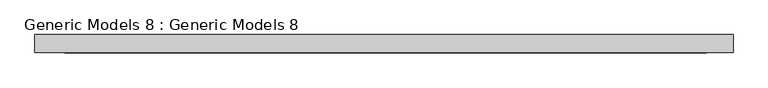
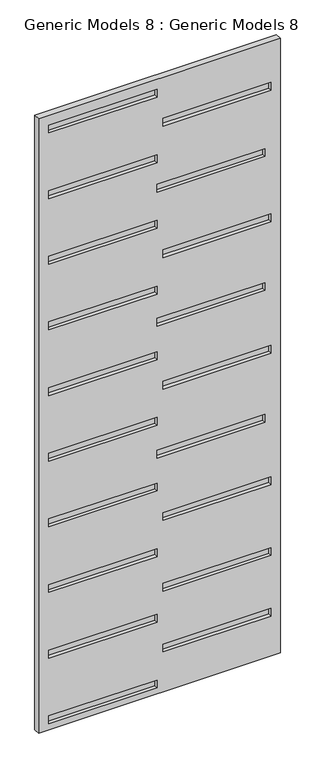
"""IFC4 building model written with IfcOpenShell, lengths in millimetres: proxy geometry, Generic Models 8 : Generic Models 8."""

from ifc_helpers import new_model, si_unit, origin, place, context, project, spatial, faceted_brep, source, transform, mapped, element, save


def generic_models_8_generic_models_8_98324a9d(model_context):
    return source(origin(), model_context, "Body", "Brep", [
        faceted_brep([(-3859.560819, -4187.674389, 7924.8), (-6812.6326914, -4187.674389, 7924.8), (-6812.6326914, -4187.674389, 0.0), (-3859.560819, -4187.674389, 0.0), (-5364.8326914, -4187.674389, 7797.8), (-5364.8326914, -4187.674389, 7696.2), (-6685.6326914, -4187.674389, 7696.2), (-6685.6326914, -4187.674389, 7797.8), (-5364.8326914, -4187.674389, 177.8), (-5364.8326914, -4187.674389, 76.2), (-6685.6326914, -4187.674389, 76.2), (-6685.6326914, -4187.674389, 177.8), (-5364.8326914, -4187.674389, 6951.1333333), (-5364.8326914, -4187.674389, 6849.5333333), (-6685.6326914, -4187.674389, 6849.5333333), (-6685.6326914, -4187.674389, 6951.1333333), (-5364.8326914, -4187.674389, 6104.4666667), (-5364.8326914, -4187.674389, 6002.8666667), (-6685.6326914, -4187.674389, 6002.8666667), (-6685.6326914, -4187.674389, 6104.4666667), (-5364.8326914, -4187.674389, 5257.8), (-5364.8326914, -4187.674389, 5156.2), (-6685.6326914, -4187.674389, 5156.2), (-6685.6326914, -4187.674389, 5257.8), (-5364.8326914, -4187.674389, 4411.1333333), (-5364.8326914, -4187.674389, 4309.5333333), (-6685.6326914, -4187.674389, 4309.5333333), (-6685.6326914, -4187.674389, 4411.1333333), (-5364.8326914, -4187.674389, 3564.4666667), (-5364.8326914, -4187.674389, 3462.8666667), (-6685.6326914, -4187.674389, 3462.8666667), (-6685.6326914, -4187.674389, 3564.4666667), (-5364.8326914, -4187.674389, 2717.8), (-5364.8326914, -4187.674389, 2616.2), (-6685.6326914, -4187.674389, 2616.2), (-6685.6326914, -4187.674389, 2717.8), (-5364.8326914, -4187.674389, 1871.1333333), (-5364.8326914, -4187.674389, 1769.5333333), (-6685.6326914, -4187.674389, 1769.5333333), (-6685.6326914, -4187.674389, 1871.1333333), (-5364.8326914, -4187.674389, 1024.4666667), (-5364.8326914, -4187.674389, 922.8666667), (-6685.6326914, -4187.674389, 922.8666667), (-6685.6326914, -4187.674389, 1024.4666667), (-3973.118008, -4187.674389, 7398.7322362), (-3973.118008, -4187.674389, 7297.1322362), (-5293.918008, -4187.674389, 7297.1322362), (-5293.918008, -4187.674389, 7398.7322362), (-3973.118008, -4187.674389, 616.9322362), (-3973.118008, -4187.674389, 515.3322362), (-5293.918008, -4187.674389, 515.3322362), (-5293.918008, -4187.674389, 616.9322362), (-3973.118008, -4187.674389, 5703.2822362), (-3973.118008, -4187.674389, 5601.6822362), (-5293.918008, -4187.674389, 5601.6822362), (-5293.918008, -4187.674389, 5703.2822362), (-3973.118008, -4187.674389, 4007.8322362), (-3973.118008, -4187.674389, 3906.2322362), (-5293.918008, -4187.674389, 3906.2322362), (-5293.918008, -4187.674389, 4007.8322362), (-3973.118008, -4187.674389, 2312.3822362), (-3973.118008, -4187.674389, 2210.7822362), (-5293.918008, -4187.674389, 2210.7822362), (-5293.918008, -4187.674389, 2312.3822362), (-4046.1719516, -4187.674389, 4842.8426322), (-4046.1719516, -4187.674389, 4741.2426322), (-5366.9719516, -4187.674389, 4741.2426322), (-5366.9719516, -4187.674389, 4842.8426322), (-4046.1719516, -4187.674389, 6570.0426322), (-4046.1719516, -4187.674389, 6468.4426322), (-5366.9719516, -4187.674389, 6468.4426322), (-5366.9719516, -4187.674389, 6570.0426322), (-4046.1719516, -4187.674389, 3141.0426322), (-4046.1719516, -4187.674389, 3039.4426322), (-5366.9719516, -4187.674389, 3039.4426322), (-5366.9719516, -4187.674389, 3141.0426322), (-3973.118008, -4187.674389, 1397.9822362), (-3973.118008, -4187.674389, 1296.3822362), (-5293.918008, -4187.674389, 1296.3822362), (-5293.918008, -4187.674389, 1397.9822362), (-3859.560819, -4111.474389, 7924.8), (-3859.560819, -4111.474389, 0.0), (-6812.6326914, -4111.474389, 0.0), (-6812.6326914, -4111.474389, 7924.8), (-5364.8326914, -4142.4938017, 7797.8), (-6685.6326914, -4142.4938017, 7797.8), (-6685.6326914, -4142.4938017, 7696.2), (-5364.8326914, -4142.4938017, 7696.2), (-5364.8326914, -4142.4938017, 177.8), (-6685.6326914, -4142.4938017, 177.8), (-6685.6326914, -4142.4938017, 76.2), (-5364.8326914, -4142.4938017, 76.2), (-5364.8326914, -4142.4938017, 6951.1333333), (-6685.6326914, -4142.4938017, 6951.1333333), (-6685.6326914, -4142.4938017, 6849.5333333), (-5364.8326914, -4142.4938017, 6849.5333333), (-5364.8326914, -4142.4938017, 6104.4666667), (-6685.6326914, -4142.4938017, 6104.4666667), (-6685.6326914, -4142.4938017, 6002.8666667), (-5364.8326914, -4142.4938017, 6002.8666667), (-5364.8326914, -4142.4938017, 5257.8), (-6685.6326914, -4142.4938017, 5257.8), (-6685.6326914, -4142.4938017, 5156.2), (-5364.8326914, -4142.4938017, 5156.2), (-5364.8326914, -4142.4938017, 4411.1333333), (-6685.6326914, -4142.4938017, 4411.1333333), (-6685.6326914, -4142.4938017, 4309.5333333), (-5364.8326914, -4142.4938017, 4309.5333333), (-5364.8326914, -4142.4938017, 3564.4666667), (-6685.6326914, -4142.4938017, 3564.4666667), (-6685.6326914, -4142.4938017, 3462.8666667), (-5364.8326914, -4142.4938017, 3462.8666667), (-5364.8326914, -4142.4938017, 2717.8), (-6685.6326914, -4142.4938017, 2717.8), (-6685.6326914, -4142.4938017, 2616.2), (-5364.8326914, -4142.4938017, 2616.2), (-5364.8326914, -4142.4938017, 1871.1333333), (-6685.6326914, -4142.4938017, 1871.1333333), (-6685.6326914, -4142.4938017, 1769.5333333), (-5364.8326914, -4142.4938017, 1769.5333333), (-5364.8326914, -4142.4938017, 1024.4666667), (-6685.6326914, -4142.4938017, 1024.4666667), (-6685.6326914, -4142.4938017, 922.8666667), (-5364.8326914, -4142.4938017, 922.8666667), (-3973.118008, -4142.4938017, 7398.7322362), (-5293.918008, -4142.4938017, 7398.7322362), (-5293.918008, -4142.4938017, 7297.1322362), (-3973.118008, -4142.4938017, 7297.1322362), (-3973.118008, -4142.4938017, 616.9322362), (-5293.918008, -4142.4938017, 616.9322362), (-5293.918008, -4142.4938017, 515.3322362), (-3973.118008, -4142.4938017, 515.3322362), (-3973.118008, -4142.4938017, 5703.2822362), (-5293.918008, -4142.4938017, 5703.2822362), (-5293.918008, -4142.4938017, 5601.6822362), (-3973.118008, -4142.4938017, 5601.6822362), (-3973.118008, -4142.4938017, 4007.8322362), (-5293.918008, -4142.4938017, 4007.8322362), (-5293.918008, -4142.4938017, 3906.2322362), (-3973.118008, -4142.4938017, 3906.2322362), (-3973.118008, -4142.4938017, 2312.3822362), (-5293.918008, -4142.4938017, 2312.3822362), (-5293.918008, -4142.4938017, 2210.7822362), (-3973.118008, -4142.4938017, 2210.7822362), (-4046.1719516, -4142.4938017, 4842.8426322), (-5366.9719516, -4142.4938017, 4842.8426322), (-5366.9719516, -4142.4938017, 4741.2426322), (-4046.1719516, -4142.4938017, 4741.2426322), (-4046.1719516, -4142.4938017, 6570.0426322), (-5366.9719516, -4142.4938017, 6570.0426322), (-5366.9719516, -4142.4938017, 6468.4426322), (-4046.1719516, -4142.4938017, 6468.4426322), (-4046.1719516, -4142.4938017, 3141.0426322), (-5366.9719516, -4142.4938017, 3141.0426322), (-5366.9719516, -4142.4938017, 3039.4426322), (-4046.1719516, -4142.4938017, 3039.4426322), (-3973.118008, -4142.4938017, 1397.9822362), (-5293.918008, -4142.4938017, 1397.9822362), (-5293.918008, -4142.4938017, 1296.3822362), (-3973.118008, -4142.4938017, 1296.3822362)], [[[0, 1, 2, 3], [4, 5, 6, 7], [8, 9, 10, 11], [12, 13, 14, 15], [16, 17, 18, 19], [20, 21, 22, 23], [24, 25, 26, 27], [28, 29, 30, 31], [32, 33, 34, 35], [36, 37, 38, 39], [40, 41, 42, 43], [44, 45, 46, 47], [48, 49, 50, 51], [52, 53, 54, 55], [56, 57, 58, 59], [60, 61, 62, 63], [64, 65, 66, 67], [68, 69, 70, 71], [72, 73, 74, 75], [76, 77, 78, 79]], [[80, 81, 82, 83]], [[1, 0, 80, 83]], [[2, 1, 83, 82]], [[3, 2, 82, 81]], [[0, 3, 81, 80]], [[84, 85, 86, 87]], [[84, 87, 5, 4]], [[87, 86, 6, 5]], [[86, 85, 7, 6]], [[85, 84, 4, 7]], [[88, 89, 90, 91]], [[88, 91, 9, 8]], [[91, 90, 10, 9]], [[90, 89, 11, 10]], [[89, 88, 8, 11]], [[92, 93, 94, 95]], [[92, 95, 13, 12]], [[95, 94, 14, 13]], [[94, 93, 15, 14]], [[93, 92, 12, 15]], [[96, 97, 98, 99]], [[96, 99, 17, 16]], [[99, 98, 18, 17]], [[98, 97, 19, 18]], [[97, 96, 16, 19]], [[100, 101, 102, 103]], [[100, 103, 21, 20]], [[103, 102, 22, 21]], [[102, 101, 23, 22]], [[101, 100, 20, 23]], [[104, 105, 106, 107]], [[104, 107, 25, 24]], [[107, 106, 26, 25]], [[106, 105, 27, 26]], [[105, 104, 24, 27]], [[108, 109, 110, 111]], [[108, 111, 29, 28]], [[111, 110, 30, 29]], [[110, 109, 31, 30]], [[109, 108, 28, 31]], [[112, 113, 114, 115]], [[112, 115, 33, 32]], [[115, 114, 34, 33]], [[114, 113, 35, 34]], [[113, 112, 32, 35]], [[116, 117, 118, 119]], [[116, 119, 37, 36]], [[119, 118, 38, 37]], [[118, 117, 39, 38]], [[117, 116, 36, 39]], [[120, 121, 122, 123]], [[120, 123, 41, 40]], [[123, 122, 42, 41]], [[122, 121, 43, 42]], [[121, 120, 40, 43]], [[124, 125, 126, 127]], [[124, 127, 45, 44]], [[127, 126, 46, 45]], [[126, 125, 47, 46]], [[125, 124, 44, 47]], [[128, 129, 130, 131]], [[128, 131, 49, 48]], [[131, 130, 50, 49]], [[130, 129, 51, 50]], [[129, 128, 48, 51]], [[132, 133, 134, 135]], [[132, 135, 53, 52]], [[135, 134, 54, 53]], [[134, 133, 55, 54]], [[133, 132, 52, 55]], [[136, 137, 138, 139]], [[136, 139, 57, 56]], [[139, 138, 58, 57]], [[138, 137, 59, 58]], [[137, 136, 56, 59]], [[140, 141, 142, 143]], [[140, 143, 61, 60]], [[143, 142, 62, 61]], [[142, 141, 63, 62]], [[141, 140, 60, 63]], [[144, 145, 146, 147]], [[144, 147, 65, 64]], [[147, 146, 66, 65]], [[146, 145, 67, 66]], [[145, 144, 64, 67]], [[148, 149, 150, 151]], [[148, 151, 69, 68]], [[151, 150, 70, 69]], [[150, 149, 71, 70]], [[149, 148, 68, 71]], [[152, 153, 154, 155]], [[152, 155, 73, 72]], [[155, 154, 74, 73]], [[154, 153, 75, 74]], [[153, 152, 72, 75]], [[156, 157, 158, 159]], [[156, 159, 77, 76]], [[159, 158, 78, 77]], [[158, 157, 79, 78]], [[157, 156, 76, 79]]]),
    ])


if __name__ == "__main__":
    model = new_model("IFC4")
    model_context = context("Model", 3, world=origin())
    ifc_project = project(units=[si_unit("LENGTHUNIT", "METRE", prefix="MILLI")], contexts=[model_context])
    site = spatial("IfcSite", under=ifc_project)
    building = spatial("IfcBuilding", under=site)
    placement = place(None, origin())
    generic_models_8_generic_models_8_shape = generic_models_8_generic_models_8_98324a9d(model_context)
    element("IfcBuildingElementProxy", 1, Name="Generic Models 8 : Generic Models 8", ObjectType="Generic Models 8 : Generic Models 8", at=placement, inside=building, context=model_context, shape_type="MappedRepresentation", body=[
        mapped(generic_models_8_generic_models_8_shape, transform((0.0, 0.0, 0.0), x_axis=(1.0, 0.0, 0.0), y_axis=(0.0, 1.0, 0.0), z_axis=(0.0, 0.0, 1.0))),
    ])
    save(model, "model.ifc")
